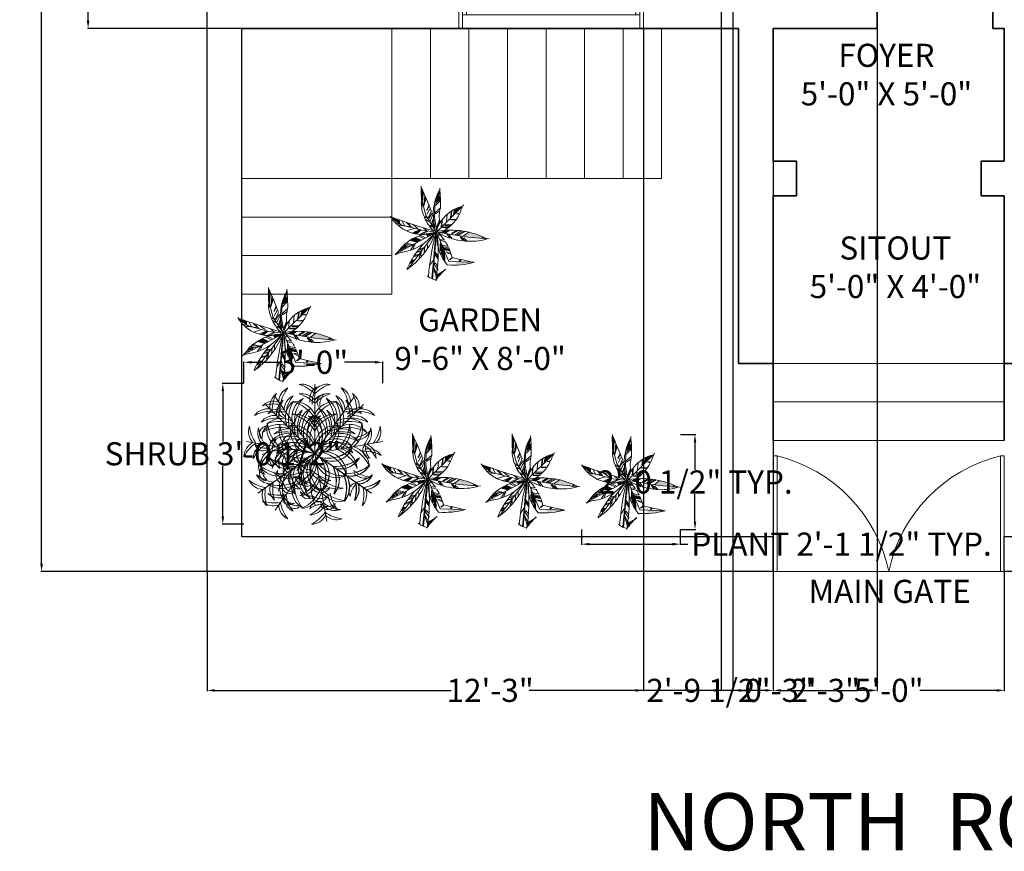
# Model space of a CAD drawing. Units: inches. Extents: x 84 to 590, y 32 to 648.
# Tile 1 of 6: x 84 to 340, y 32 to 248. Entities that reach past the tile are written whole.
import ezdxf

# ---------------------------------------------------------------- set-up
doc = ezdxf.new("R2010")
doc.units = ezdxf.units.IN
doc.header["$MEASUREMENT"] = 0
for name, color, linetype, lineweight in [('A-ANNO-DIMS', 2, 'Continuous', 18), ('A-ANNO-TEXT', 7, 'Continuous', 18), ('A-AREA-IDEN', 7, 'Continuous', 18), ('A-DOOR', 4, 'Continuous', 18), ('A-FLOR-STRS', 7, 'Continuous', 18), ('A-GLAZ', 4, 'Continuous', 18), ('A-WALL', 7, 'Continuous', 35), ('C-PROP', 7, 'Continuous', 30), ('L-PLNT', 3, 'Continuous', 13)]:
    doc.layers.add(name, color=color, linetype=linetype, lineweight=lineweight)
doc.styles.get("Standard").update_dxf_attribs({"font": 'arial.ttf'})
doc.dimstyles.get("Standard").update_dxf_attribs({"dimtxt": 6, "dimasz": 2, "dimexe": 0.18, "dimexo": 0.0625, "dimgap": 0.09, "dimtad": 0, "dimtih": 1, "dimtoh": 1, "dimdec": 0, "dimzin": 0, "dimdsep": 46, "dimlunit": 4, "dimtxsty": 'Standard', "dimcen": 0.09, "dimadec": 0, "dimazin": 0, "dimtfac": 1, "dimtdec": 0, "dimtofl": 0, "dimtmove": 0, "dimatfit": 3, "dimfxl": 1, "dimtolj": 1, "dimtzin": 0, "dimarcsym": 1})

# ---------------------------------------------------------------- blocks, each defined once
blk = doc.blocks.new('DOOR')
for p, q in [((185.51, 1128.53), (185.51, 1098.53)), ((185.51, 1128.53), (186.51, 1128.53)), ((186.51, 1098.53), (186.51, 1128.53)), ((186.51, 1098.53), (156.51, 1098.53))]:
    blk.add_line(p, q)
blk.add_arc((194.73, 1090.6), 39.03, 103.6607, 168.2814)
blk = doc.blocks.new('A$C5D061C3B')
for p, q in [((3.377, 6.679), (3.377, 3.377)), ((1.03, 5.716), (3.365, 3.381)), ((1.483, 6.082), (3.377, 3.377)), ((5.259, 6.086), (3.365, 3.381)), ((5.712, 5.712), (3.377, 3.377)), ((0.125, 3.951), (3.377, 3.377)), ((6.629, 3.951), (3.377, 3.377)), ((0.66, 1.487), (3.365, 3.381)), ((1.483, 0.672), (3.377, 3.377)), ((6.07, 1.487), (3.365, 3.381)), ((3.951, 0.125), (3.377, 3.377)), ((6.082, 1.483), (3.377, 3.377))]:
    blk.add_line(p, q)
for centre, radius, start, end in [((2.763, 5.924), 0.762, 36.29, 99.6243), ((2.145, 5.032), 1.715, 44.0763, 73.3794), ((3.991, 5.924), 0.762, 80.3757, 143.71), ((4.61, 5.032), 1.715, 106.6206, 135.9237), ((1.998, 5.617), 0.762, 125.3757, 188.71), ((3.066, 5.423), 1.715, 151.6206, 180.9237), ((2.419, 5.816), 0.762, 115.3757, 178.71), ((3.438, 5.44), 1.715, 141.6206, 170.9237), ((2.678, 5.447), 0.762, 115.3757, 178.71), ((3.696, 5.07), 1.715, 141.6206, 170.9237), ((2.763, 5.474), 0.762, 36.29, 99.6243), ((2.145, 4.581), 1.715, 44.0763, 73.3794), ((3.901, 5.939), 0.762, 125.3757, 188.71), ((4.969, 5.745), 1.715, 151.6206, 180.9237), ((3.991, 5.474), 0.762, 80.3757, 143.71), ((4.61, 4.581), 1.715, 106.6206, 135.9237), ((3.871, 5.832), 0.38, 94.742, 213.7475), ((4.447, 5.681), 0.826, 139.618, 183.2106), ((4.064, 5.451), 0.762, 1.29, 64.6243), ((3.046, 5.075), 1.715, 9.0763, 38.3794), ((3.305, 5.444), 1.715, 9.0763, 38.3794), ((4.323, 5.82), 0.762, 1.29, 64.6243), ((4.744, 5.613), 0.762, 351.29, 54.6243), ((3.676, 5.419), 1.715, 359.0763, 28.3794), ((1.413, 5.111), 0.762, 71.29, 134.6243), ((1.419, 4.026), 1.715, 79.0763, 108.3794), ((2.317, 5.298), 0.762, 125.3757, 188.71), ((1.991, 5.462), 0.38, 139.742, 258.7475), ((3.385, 5.104), 1.715, 151.6206, 180.9237), ((2.505, 5.763), 0.826, 184.618, 228.2106), ((3.035, 5.062), 1.056, 129.6063, 199.7511), ((3.894, 4.989), 1.77, 149.9634, 193.6288), ((3.344, 5.089), 1.056, 119.6063, 189.7511), ((2.422, 4.799), 1.056, 25.2489, 95.3937), ((1.866, 4.14), 1.77, 31.3712, 75.0366), ((4.177, 4.869), 1.77, 139.9634, 183.6288), ((4.332, 4.799), 1.056, 84.6063, 154.7511), ((4.888, 4.14), 1.77, 104.9634, 148.6288), ((3.398, 5.094), 1.056, 350.2489, 60.3937), ((2.565, 4.873), 1.77, 356.3712, 40.0366), ((2.848, 4.985), 1.77, 346.3712, 30.0366), ((3.707, 5.058), 1.056, 340.2489, 50.3937), ((3.357, 5.1), 1.715, 359.0763, 28.3794), ((4.425, 5.294), 0.762, 351.29, 54.6243), ((1.13, 4.748), 0.762, 81.29, 144.6243), ((1.324, 3.68), 1.715, 89.0763, 118.3794), ((1.448, 4.43), 0.762, 81.29, 144.6243), ((1.671, 4.742), 0.762, 71.29, 134.6243), ((1.677, 3.657), 1.715, 79.0763, 108.3794), ((2.422, 4.198), 1.056, 25.2489, 95.3937), ((1.866, 3.54), 1.77, 31.3712, 75.0366), ((3.46, 4.637), 1.056, 129.6063, 199.7511), ((4.319, 4.565), 1.77, 149.9634, 193.6288), ((3.688, 4.597), 1.056, 119.6063, 189.7511), ((4.522, 4.377), 1.77, 139.9634, 183.6288), ((3.868, 4.321), 1.029, 121.3654, 221.5741), ((4.556, 4.237), 1.557, 141.8122, 203.3335), ((4.035, 4.215), 1.029, 111.3654, 211.5741), ((2.707, 4.219), 1.029, 328.4259, 68.6346), ((2.044, 4.017), 1.557, 346.6665, 48.1878), ((4.698, 4.013), 1.557, 131.8122, 193.3335), ((4.332, 4.198), 1.056, 84.6063, 154.7511), ((4.888, 3.54), 1.77, 104.9634, 148.6288), ((2.187, 4.233), 1.557, 336.6665, 38.1878), ((2.875, 4.316), 1.029, 318.4259, 58.6346), ((2.221, 4.381), 1.77, 356.3712, 40.0366), ((3.054, 4.602), 1.056, 350.2489, 60.3937), ((3.283, 4.633), 1.056, 340.2489, 50.3937), ((2.424, 4.56), 1.77, 346.3712, 30.0366), ((5.065, 3.661), 1.715, 71.6206, 100.9237), ((5.071, 4.746), 0.762, 45.3757, 108.71), ((5.564, 4.807), 0.762, 80.3757, 143.71), ((6.182, 3.914), 1.715, 106.6206, 135.9237), ((5.294, 4.425), 0.762, 35.3757, 98.71), ((5.419, 3.676), 1.715, 61.6206, 90.9237), ((5.613, 4.744), 0.762, 35.3757, 98.71), ((1.642, 3.362), 1.715, 89.0763, 118.3794), ((1.685, 3.712), 1.056, 70.2489, 140.3937), ((2.143, 4.564), 1.056, 164.6063, 234.7511), ((1.78, 3.994), 1.056, 60.2489, 130.3937), ((1.702, 3.136), 1.77, 66.3712, 110.0366), ((2.888, 4.998), 1.77, 184.9634, 228.6288), ((2.734, 4.46), 1.056, 164.6063, 234.7511), ((3.48, 4.893), 1.77, 184.9634, 228.6288), ((2.358, 3.686), 1.029, 3.4259, 103.6346), ((3.25, 4.435), 1.029, 156.3654, 256.5741), ((3.862, 4.761), 1.557, 176.8122, 238.3335), ((4.397, 3.686), 1.029, 76.3654, 176.5741), ((2.893, 4.761), 1.557, 301.6665, 3.1878), ((3.504, 4.435), 1.029, 283.4259, 23.6346), ((5.04, 3.14), 1.77, 69.9634, 113.6288), ((4.963, 3.998), 1.056, 49.6063, 119.7511), ((3.275, 4.893), 1.77, 311.3712, 355.0366), ((4.02, 4.46), 1.056, 305.2489, 15.3937), ((5.058, 3.707), 1.056, 39.6063, 109.7511), ((3.866, 4.998), 1.77, 311.3712, 355.0366), ((5.1, 3.357), 1.715, 61.6206, 90.9237), ((4.611, 4.564), 1.056, 305.2489, 15.3937), ((0.975, 4.424), 0.762, 160.3757, 223.71), ((1.962, 4.878), 1.715, 186.6206, 215.9237), ((1.419, 4.346), 0.762, 160.3757, 223.71), ((2.405, 4.8), 1.715, 186.6206, 215.9237), ((1.12, 4.31), 0.38, 94.742, 213.7475), ((1.696, 4.159), 0.826, 139.618, 183.2106), ((1.757, 2.853), 1.77, 76.3712, 120.0366), ((2.109, 3.287), 1.056, 70.2489, 140.3937), ((2.124, 3.502), 1.056, 60.2489, 130.3937), ((2.046, 2.644), 1.77, 66.3712, 110.0366), ((2.387, 3.752), 0.574, 99.9865, 199.4034), ((3.599, 3.314), 1.651, 142.5759, 170.8942), ((1.93, 3.14), 1.557, 21.6665, 83.1878), ((4.824, 3.14), 1.557, 96.8122, 158.3335), ((4.696, 2.648), 1.77, 69.9634, 113.6288), ((4.618, 3.506), 1.056, 49.6063, 119.7511), ((4.633, 3.283), 1.056, 39.6063, 109.7511), ((4.985, 2.848), 1.77, 59.9634, 103.6288), ((4.988, 5.812), 1.715, 279.0763, 308.3794), ((5.365, 4.794), 0.762, 271.29, 334.6243), ((4.349, 4.8), 1.715, 324.0763, 353.3794), ((5.335, 4.346), 0.762, 316.29, 19.6243), ((4.793, 4.878), 1.715, 324.0763, 353.3794), ((5.779, 4.424), 0.762, 316.29, 19.6243), ((0.762, 3.214), 0.762, 116.29, 179.6243), ((1.534, 2.451), 1.715, 124.0763, 153.3794), ((1.206, 3.136), 0.762, 116.29, 179.6243), ((1.977, 2.373), 1.715, 124.0763, 153.3794), ((1.062, 4.452), 0.826, 229.618, 273.2106), ((0.91, 3.875), 0.38, 184.742, 303.7475), ((1.588, 3.666), 0.38, 94.742, 213.7475), ((2.182, 2.428), 1.77, 76.3712, 120.0366), ((2.165, 3.515), 0.826, 139.618, 183.2106), ((2.426, 2.879), 1.029, 48.4259, 148.6346), ((2.365, 3.045), 1.029, 38.4259, 138.6346), ((2.328, 2.353), 1.557, 56.6665, 118.1878), ((2.84, 3.739), 0.372, 69.2257, 210.1279), ((3.109, 3.59), 0.515, 105.4398, 183.6694), ((4.414, 2.358), 1.557, 61.8122, 123.3335), ((4.377, 3.05), 1.029, 41.3654, 141.5741), ((4.316, 2.875), 1.029, 31.3654, 131.5741), ((4.56, 2.424), 1.77, 59.9634, 103.6288), ((4.777, 2.373), 1.715, 26.6206, 55.9237), ((5.549, 3.136), 0.762, 0.3757, 63.71), ((1.811, 2.684), 1.056, 105.2489, 175.3937), ((2.363, 2.022), 1.77, 111.3712, 155.0366), ((2.185, 0.015), 3.567, 70.4772, 111.6585), ((1.447, 3.129), 0.376, 122.0577, 257.8533), ((1.751, 3.126), 0.529, 140.1845, 223.654), ((2.403, 2.58), 1.056, 105.2489, 175.3937), ((2.955, 1.917), 1.77, 111.3712, 155.0366), ((2.007, 3.071), 0.506, 93.8744, 233.9763), ((2.51, 2.191), 1.557, 66.6665, 128.1878), ((2.729, 4.702), 1.557, 221.8122, 283.3335), ((2.527, 4.039), 1.029, 201.3654, 301.5741), ((4.912, 0.157), 3.567, 115.4772, 156.6585), ((2.489, 2.932), 0.825, 128.7536, 199.097), ((2.896, 2.427), 1.029, 83.4259, 183.6346), ((3.359, 1.911), 1.557, 101.6665, 163.1878), ((2.903, 2.8), 0.855, 116.4477, 194.3672), ((4.744, 1.779), 2.789, 140.4007, 163.139), ((2.741, 3.253), 0.372, 114.2257, 255.1279), ((3.037, 3.338), 0.515, 150.4398, 228.6694), ((6.727, 2.189), 3.567, 160.4772, 201.6585), ((4.233, 2.187), 1.557, 51.8122, 113.3335), ((4.001, 4.702), 1.557, 256.6665, 318.1878), ((4.013, 4.698), 1.557, 256.6665, 318.1878), ((4.203, 4.039), 1.029, 238.4259, 338.6346), ((4.215, 4.035), 1.029, 238.4259, 338.6346), ((3.395, 1.911), 1.557, 16.8122, 78.3335), ((3.858, 2.427), 1.029, 356.3654, 96.5741), ((3.799, 1.917), 1.77, 24.9634, 68.6288), ((4.352, 2.58), 1.056, 4.6063, 74.7511), ((4.391, 2.022), 1.77, 24.9634, 68.6288), ((4.943, 2.684), 1.056, 4.6063, 74.7511), ((6.053, 3.533), 0.38, 146.2525, 265.258), ((5.741, 1.774), 1.715, 61.6206, 90.9237), ((6.629, 3.684), 0.826, 176.7894, 220.382), ((5.935, 2.842), 0.762, 35.3757, 98.71), ((1.067, 2.749), 0.376, 122.0577, 257.8533), ((1.873, 4.181), 1.77, 229.9634, 273.6288), ((1.653, 3.348), 1.056, 209.6063, 279.7511), ((1.37, 2.745), 0.529, 140.1845, 223.654), ((2.145, 3.693), 1.056, 209.6063, 279.7511), ((2.365, 4.526), 1.77, 229.9634, 273.6288), ((2.328, 4.401), 1.557, 241.8122, 303.3335), ((2.365, 3.709), 1.029, 221.3654, 321.5741), ((2.412, 2.943), 0.574, 144.9865, 244.4034), ((3.578, 3.49), 1.651, 187.5759, 215.8942), ((1.911, 3.359), 1.557, 286.8122, 348.3335), ((2.427, 2.896), 1.029, 266.3654, 6.5741), ((3.45, 2.634), 0.855, 161.4477, 239.3672), ((3.003, 2.844), 0.372, 159.2257, 300.1279), ((3.152, 3.113), 0.515, 195.4398, 273.6694), ((3.697, 2.369), 1.029, 128.4259, 228.6346), ((5.474, 3.214), 2.789, 185.4007, 208.139), ((4.389, 2.332), 1.557, 146.6665, 208.1878), ((4.035, 2.539), 1.029, 148.4259, 248.6346), ((4.698, 2.741), 1.557, 166.6665, 228.1878), ((4.435, 3.25), 1.029, 193.4259, 293.6346), ((4.761, 3.862), 1.557, 211.6665, 273.1878), ((2.341, 2.332), 1.557, 331.8122, 33.3335), ((2.353, 2.328), 1.557, 331.8122, 33.3335), ((3.033, 2.369), 1.029, 311.3654, 51.5741), ((3.045, 2.365), 1.029, 311.3654, 51.5741), ((4.365, 4.526), 1.77, 266.3712, 310.0366), ((4.377, 4.522), 1.77, 266.3712, 310.0366), ((4.585, 3.693), 1.056, 260.2489, 330.3937), ((4.597, 3.688), 1.056, 260.2489, 330.3937), ((4.857, 4.181), 1.77, 266.3712, 310.0366), ((4.869, 4.177), 1.77, 266.3712, 310.0366), ((5.077, 3.348), 1.056, 260.2489, 330.3937), ((5.089, 3.344), 1.056, 260.2489, 330.3937), ((1.672, 3.7), 1.715, 231.6206, 260.9237), ((1.295, 2.682), 0.762, 205.3757, 268.71), ((1.122, 2.441), 0.38, 139.742, 258.7475), ((1.636, 2.741), 0.826, 184.618, 228.2106), ((2.046, 4.111), 1.77, 249.9634, 293.6288), ((2.124, 3.252), 1.056, 229.6063, 299.7511), ((1.908, 2.317), 0.38, 139.742, 258.7475), ((2.422, 2.617), 0.826, 184.618, 228.2106), ((3.607, 1.706), 1.77, 156.3712, 200.0366), ((2.624, 2.192), 0.506, 138.8744, 278.9763), ((3.24, 2.128), 1.056, 150.2489, 220.3937), ((3.064, 2.435), 0.825, 173.7536, 244.097), ((4.099, 2.051), 1.77, 156.3712, 200.0366), ((4.522, 2.378), 1.77, 176.3712, 220.0366), ((3.942, 2.908), 0.855, 206.4477, 284.3672), ((4.963, 4.749), 2.789, 230.4007, 253.139), ((2.632, 2.051), 1.77, 339.9634, 23.6288), ((2.644, 2.046), 1.77, 339.9634, 23.6288), ((3.49, 2.128), 1.056, 319.6063, 29.7511), ((3.502, 2.124), 1.056, 319.6063, 29.7511), ((3.124, 1.706), 1.77, 339.9634, 23.6288), ((3.136, 1.702), 1.77, 339.9634, 23.6288), ((6.244, 3.948), 1.715, 234.0763, 263.3794), ((5.79, 2.962), 0.762, 226.29, 289.6243), ((5.058, 3.7), 1.715, 279.0763, 308.3794), ((5.07, 3.696), 1.715, 279.0763, 308.3794), ((5.435, 2.682), 0.762, 271.29, 334.6243), ((5.447, 2.678), 0.762, 271.29, 334.6243), ((0.926, 2.424), 0.762, 205.3757, 268.71), ((1.303, 3.442), 1.715, 231.6206, 260.9237), ((1.702, 3.619), 1.77, 249.9634, 293.6288), ((1.78, 2.76), 1.056, 229.6063, 299.7511), ((2, 1.676), 0.762, 161.29, 224.6243), ((3.086, 1.681), 1.715, 169.0763, 198.3794), ((2.748, 1.784), 1.056, 150.2489, 220.3937), ((2.188, 1.837), 0.376, 167.0577, 302.8533), ((2.405, 2.049), 0.529, 185.1845, 268.654), ((4.177, 1.886), 1.77, 176.3712, 220.0366), ((3.428, 3.603), 1.651, 232.5759, 260.8942), ((2.99, 2.391), 0.574, 189.9865, 289.4034), ((3.688, 2.157), 1.056, 170.2489, 240.3937), ((1.917, 2.955), 1.77, 294.9634, 338.6288), ((2.58, 2.403), 1.056, 274.6063, 344.7511), ((3.81, 2.493), 0.825, 218.7536, 289.097), ((3.671, 2.011), 0.506, 183.8744, 323.9763), ((4.893, 3.48), 1.77, 221.3712, 265.0366), ((4.46, 2.734), 1.056, 215.2489, 285.3937), ((3.982, 1.784), 1.056, 319.6063, 29.7511), ((3.994, 1.78), 1.056, 319.6063, 29.7511), ((5.385, 1.584), 0.38, 101.2525, 220.258), ((5.899, 1.283), 0.826, 131.7894, 175.382), ((3.645, 1.681), 1.715, 341.6206, 10.9237), ((4.73, 1.676), 0.762, 315.3757, 18.71), ((3.657, 1.677), 1.715, 341.6206, 10.9237), ((4.742, 1.671), 0.762, 315.3757, 18.71), ((5.427, 3.442), 1.715, 279.0763, 308.3794), ((5.44, 3.438), 1.715, 279.0763, 308.3794), ((5.804, 2.424), 0.762, 271.29, 334.6243), ((5.816, 2.419), 0.762, 271.29, 334.6243), ((1.631, 1.417), 0.762, 161.29, 224.6243), ((2.717, 1.423), 1.715, 169.0763, 198.3794), ((1.671, 2.012), 0.762, 225.3757, 288.71), ((1.677, 3.098), 1.715, 251.6206, 280.9237), ((2.405, 1.511), 0.529, 185.1845, 268.654), ((3.696, 1.684), 1.715, 189.0763, 218.3794), ((3.344, 1.665), 1.056, 170.2489, 240.3937), ((3.227, 2.169), 0.826, 229.618, 273.2106), ((3.076, 1.593), 0.38, 184.742, 303.7475), ((2.022, 2.363), 1.77, 294.9634, 338.6288), ((2.684, 1.811), 1.056, 274.6063, 344.7511), ((4.998, 2.888), 1.77, 221.3712, 265.0366), ((4.564, 2.143), 1.056, 215.2489, 285.3937), ((5.808, 1.754), 1.715, 189.0763, 218.3794), ((4.014, 1.423), 1.715, 341.6206, 10.9237), ((5.099, 1.417), 0.762, 315.3757, 18.71), ((1.419, 2.729), 1.715, 251.6206, 280.9237), ((1.413, 1.643), 0.762, 225.3757, 288.71), ((3.438, 1.315), 1.715, 189.0763, 218.3794), ((2.188, 1.299), 0.376, 167.0577, 302.8533), ((2.678, 1.307), 0.762, 181.29, 244.6243), ((2.583, 1.701), 0.826, 229.618, 273.2106), ((2.432, 1.124), 0.38, 184.742, 303.7475), ((2.373, 1.977), 1.715, 296.6206, 325.9237), ((3.528, 0.69), 0.38, 56.2525, 175.258), ((3.616, 1.755), 0.529, 230.1845, 313.654), ((3.613, 1.452), 0.376, 212.0577, 347.8533), ((3.997, 1.374), 0.529, 230.1845, 313.654), ((3.994, 1.071), 0.376, 212.0577, 347.8533), ((4.8, 2.405), 1.715, 234.0763, 263.3794), ((4.79, 1.377), 0.762, 181.29, 244.6243), ((2.419, 0.938), 0.762, 181.29, 244.6243), ((3.136, 1.206), 0.762, 270.3757, 333.71), ((3.68, 0.113), 0.826, 86.7894, 130.382), ((2.451, 1.534), 1.715, 296.6206, 325.9237), ((4.346, 1.419), 0.762, 226.29, 289.6243), ((4.878, 1.962), 1.715, 234.0763, 263.3794), ((3.214, 0.762), 0.762, 270.3757, 333.71), ((4.424, 0.975), 0.762, 226.29, 289.6243)]:
    blk.add_arc(centre, radius, start, end)
blk = doc.blocks.new('A$C40F70BF2')
for p, q in [((1.395, 3.412), (1.345, 4.14)), ((1.378, 3.827), (1.371, 4.019)), ((1.386, 3.761), (1.393, 4.004)), ((1.404, 3.622), (1.407, 3.935)), ((1.411, 3.538), (1.419, 3.905)), ((1.937, 3.412), (2.147, 3.983)), ((2.077, 3.788), (2.151, 3.896)), ((1.389, 3.49), (1.353, 3.553)), ((1.393, 3.445), (1.356, 3.526)), ((1.393, 3.403), (1.356, 3.493)), ((1.411, 3.334), (1.36, 3.445)), ((1.448, 3.313), (1.496, 3.752)), ((1.529, 3.679), (1.455, 3.289)), ((1.455, 3.289), (1.55, 3.622)), ((2.18, 3.523), (1.96, 3.294)), ((1.974, 3.403), (2.165, 3.619)), ((2.165, 3.571), (1.974, 3.403)), ((1.989, 3.487), (2.151, 3.679)), ((2.165, 3.619), (1.989, 3.487)), ((2.033, 3.595), (2.135, 3.727)), ((2.151, 3.679), (2.033, 3.595)), ((2.062, 3.679), (2.135, 3.824)), ((2.135, 3.727), (2.062, 3.679)), ((2.135, 3.824), (2.077, 3.788)), ((1.43, 3.289), (1.349, 3.412)), ((1.426, 3.264), (1.353, 3.376)), ((1.536, 2.871), (1.395, 3.412)), ((1.587, 3.114), (1.683, 3.328)), ((1.591, 3.078), (1.587, 3.114)), ((1.701, 3.289), (1.591, 3.078)), ((1.606, 2.916), (1.705, 3.132)), ((1.65, 2.748), (1.785, 3.066)), ((1.919, 2.785), (1.937, 3.412)), ((1.96, 3.006), (2.18, 3.198)), ((2.151, 3.066), (1.96, 2.933)), ((2.006, 2.139), (3.105, 3.225)), ((2.626, 2.774), (2.662, 3.065)), ((2.653, 2.781), (2.685, 3.069)), ((2.797, 3.138), (2.753, 2.909)), ((2.855, 3.162), (2.797, 2.933)), ((2.797, 2.933), (2.797, 3.138)), ((2.885, 3.162), (2.826, 2.957)), ((2.826, 2.957), (2.855, 3.162)), ((2.929, 3.174), (2.855, 3.006)), ((2.855, 3.006), (2.885, 3.162)), ((2.899, 3.018), (2.929, 3.174)), ((2.944, 3.15), (2.899, 3.018)), ((2.958, 3.186), (2.929, 3.066)), ((2.929, 3.066), (2.944, 3.15)), ((2.973, 3.114), (2.958, 3.186)), ((3.002, 3.21), (2.973, 3.114)), ((3.032, 3.234), (3.002, 3.162)), ((3.002, 3.162), (3.002, 3.21)), ((0.438, 2.456), (0.018, 2.796)), ((0.505, 2.608), (0.623, 2.404)), ((1.58, 2.772), (1.451, 2.841)), ((1.472, 2.791), (1.602, 2.739)), ((1.992, 2.139), (1.536, 2.871)), ((1.538, 2.69), (1.679, 2.617)), ((1.564, 2.648), (1.679, 2.596)), ((1.602, 2.739), (1.58, 2.772)), ((1.668, 2.733), (1.65, 2.748)), ((1.822, 2.967), (1.668, 2.733)), ((1.73, 2.628), (1.844, 2.883)), ((1.789, 2.517), (1.873, 2.748)), ((1.8, 2.478), (1.88, 2.664)), ((2.024, 2.154), (1.919, 2.785)), ((1.96, 2.933), (1.96, 3.006)), ((2.216, 2.359), (2.243, 2.624)), ((2.238, 2.386), (2.257, 2.647)), ((2.446, 2.617), (2.471, 2.889)), ((2.621, 2.684), (2.895, 2.703)), ((2.621, 2.677), (2.849, 2.673)), ((2.877, 2.934), (3.045, 2.983)), ((3.008, 2.919), (2.877, 2.934)), ((0.211, 2.512), (0.476, 2.476)), ((0.314, 2.44), (0.828, 2.38)), ((1.381, 2.214), (0.438, 2.456)), ((0.696, 2.548), (0.916, 2.356)), ((0.696, 2.187), (1.034, 2.295)), ((0.916, 2.356), (0.784, 2.5)), ((0.96, 2.476), (1.196, 2.295)), ((1.269, 2.236), (0.96, 2.103)), ((1.019, 2.067), (1.269, 2.236)), ((1.078, 2.062), (1.295, 2.219)), ((1.129, 2.052), (1.321, 2.219)), ((1.313, 2.055), (1.578, 2.175)), ((1.974, 2.139), (1.381, 2.214)), ((1.387, 2.043), (1.665, 2.187)), ((1.431, 2.32), (1.592, 2.199)), ((1.789, 2.411), (1.627, 2.469)), ((1.672, 2.415), (1.811, 2.369)), ((1.811, 2.369), (1.789, 2.411)), ((2.27, 2.33), (2.289, 2.356)), ((2.498, 2.311), (2.27, 2.33)), ((2.289, 2.356), (2.58, 2.344)), ((2.366, 2.415), (2.384, 2.442)), ((2.612, 2.4), (2.366, 2.415)), ((2.369, 2.481), (2.676, 2.471)), ((2.375, 2.079), (2.567, 2.21)), ((2.384, 2.442), (2.644, 2.427)), ((2.662, 2.072), (2.881, 2.203)), ((2.699, 2.053), (2.968, 2.206)), ((2.831, 2.016), (3.118, 2.199)), ((2.913, 2.012), (3.218, 2.176)), ((3.264, 2.165), (2.977, 2.001)), ((1.974, 2.113), (0.228, 1.183)), ((1.974, 2.128), (0.802, 0.571)), ((1.225, 1.959), (1.46, 1.862)), ((1.284, 2.007), (1.504, 1.898)), ((2.003, 2.103), (1.827, 0.082)), ((1.974, 1.995), (1.915, 1.405)), ((2.006, 2.139), (2.548, 0.855)), ((2.07, 2.139), (2.758, 2.02)), ((2.083, 2.012), (2.22, 1.967)), ((2.179, 1.762), (2.156, 1.818)), ((2.156, 1.818), (2.361, 1.788)), ((2.402, 1.714), (2.179, 1.762)), ((2.548, 2.035), (2.457, 2.046)), ((2.457, 2.046), (2.603, 1.863)), ((2.69, 1.84), (2.548, 2.035)), ((2.758, 2.02), (3.387, 1.915)), ((2.977, 2.001), (2.913, 2.012)), ((3.177, 1.747), (3.041, 1.93)), ((3.041, 1.93), (3.105, 1.915)), ((3.105, 1.915), (3.255, 1.736)), ((3.168, 1.952), (3.415, 2.135)), ((3.332, 1.747), (3.196, 1.889)), ((3.387, 1.915), (3.907, 1.867)), ((3.911, 1.863), (4.308, 1.837)), ((3.975, 1.885), (4.057, 1.915)), ((4.012, 1.878), (3.975, 1.885)), ((4.085, 1.904), (4.012, 1.878)), ((0.387, 1.333), (0.505, 1.357)), ((0.417, 1.381), (0.578, 1.405)), ((0.505, 1.357), (0.417, 1.381)), ((0.461, 1.429), (0.667, 1.442)), ((0.578, 1.405), (0.461, 1.429)), ((0.476, 1.465), (0.696, 1.478)), ((0.667, 1.442), (0.476, 1.465)), ((0.696, 1.478), (0.549, 1.526)), ((0.549, 1.526), (0.814, 1.513)), ((0.814, 1.513), (0.578, 1.562)), ((0.593, 1.61), (0.902, 1.562)), ((0.96, 1.586), (0.667, 1.646)), ((0.872, 1.345), (1.019, 1.586)), ((0.902, 1.562), (0.96, 1.586)), ((0.989, 1.405), (1.093, 1.646)), ((1.206, 1.34), (1.436, 1.403)), ((1.231, 1.403), (1.462, 1.445)), ((1.475, 1.237), (1.504, 1.501)), ((1.915, 1.405), (1.871, 0.852)), ((2.175, 1.512), (2.165, 1.441)), ((2.165, 1.441), (2.165, 1.363)), ((2.179, 1.676), (2.175, 1.605)), ((2.175, 1.605), (2.175, 1.512)), ((2.179, 1.314), (2.179, 1.676)), ((2.184, 1.501), (2.179, 1.407)), ((2.179, 1.407), (2.179, 1.314)), ((2.193, 1.613), (2.184, 1.501)), ((2.197, 1.46), (2.193, 1.613)), ((2.197, 1.392), (2.197, 1.46)), ((2.206, 1.277), (2.197, 1.392)), ((2.225, 1.501), (2.211, 1.378)), ((2.211, 1.378), (2.211, 1.172)), ((2.216, 1.34), (2.225, 1.422)), ((2.216, 1.273), (2.216, 1.34)), ((2.225, 1.422), (2.225, 1.501)), ((2.238, 1.303), (2.229, 1.232)), ((2.243, 1.389), (2.238, 1.303)), ((2.247, 1.46), (2.243, 1.389)), ((2.257, 1.534), (2.247, 1.46)), ((2.257, 1.544), (2.257, 1.534)), ((2.261, 1.213), (2.261, 1.535)), ((2.298, 1.486), (2.27, 1.56)), ((2.27, 1.56), (2.521, 1.501)), ((2.279, 1.396), (2.275, 1.314)), ((2.275, 1.314), (2.275, 1.247)), ((2.289, 1.318), (2.279, 1.396)), ((2.289, 1.157), (2.289, 1.318)), ((2.302, 1.292), (2.293, 1.224)), ((2.548, 1.441), (2.298, 1.486)), ((2.307, 1.37), (2.302, 1.292)), ((2.307, 1.023), (2.307, 1.37)), ((2.334, 0.926), (2.343, 1.325)), ((2.371, 0.847), (2.357, 1.299)), ((0.843, 0.792), (0.989, 0.876)), ((0.872, 0.864), (1.049, 0.924)), ((0.989, 0.876), (0.872, 0.864)), ((1.049, 0.924), (0.931, 0.912)), ((1.019, 1.056), (1.21, 1.129)), ((1.049, 1.105), (1.24, 1.165)), ((1.254, 1.008), (1.313, 1.249)), ((1.327, 1.093), (1.342, 1.273)), ((1.709, 0.671), (1.871, 0.912)), ((1.944, 1.141), (1.944, 1.261)), ((1.944, 1.261), (2.077, 1.08)), ((2.077, 0.948), (1.944, 1.141)), ((2.062, 1.026), (1.947, 1.204)), ((2.206, 1.105), (2.206, 1.277)), ((2.211, 1.172), (2.206, 1.105)), ((2.225, 1.157), (2.216, 1.273)), ((2.229, 1.232), (2.225, 1.157)), ((2.27, 1.109), (2.261, 1.213)), ((2.275, 1.247), (2.27, 1.18)), ((2.27, 1.18), (2.27, 1.109)), ((2.293, 1.015), (2.289, 1.157)), ((2.293, 1.154), (2.289, 1.083)), ((2.289, 1.083), (2.293, 1.015)), ((2.293, 1.224), (2.293, 1.154)), ((2.311, 0.948), (2.307, 1.023)), ((2.433, 1.267), (2.637, 1.215)), ((2.471, 1.236), (2.65, 1.152)), ((2.69, 1.027), (2.571, 0.922)), ((2.699, 1.008), (2.594, 0.922)), ((3.063, 0.941), (2.995, 0.87)), ((3.095, 0.937), (3.013, 0.851)), ((0.814, 0.744), (0.96, 0.804)), ((0.96, 0.804), (0.843, 0.792)), ((1.871, 0.852), (1.798, 0.13)), ((1.886, 0.527), (1.886, 0.587)), ((1.886, 0.587), (2.003, 0.322)), ((2.003, 0.154), (1.886, 0.527)), ((1.915, 0.696), (1.93, 0.792)), ((2.077, 0.491), (1.915, 0.696)), ((1.93, 0.792), (2.062, 0.647)), ((2.548, 0.855), (3.647, 0.814))]:
    blk.add_line(p, q)
for centre, radius, start, end in [((7.228, 3.925), 5.886, 178.201, 184.8569), ((-12.631, -2.337), 15.387, 20.511, 24.7274), ((3.986, 2.93), 2.121, 151.1341, 194.9744), ((-4.468, 3.341), 6.654, 358.6497, 6.1521), ((3.081, 3.443), 1.737, 181.0191, 200.3048), ((3.488, 1.763), 1.537, 103.7474, 164.6646), ((3.323, 2.824), 1.195, 162.4534, 194.3671), ((1.484, 3.655), 1.692, 336.4968, 341.7386), ((4.255, 2.671), 1.249, 148.3784, 158.7208), ((1.388, 3.636), 1.607, 210.2718, 288.6073), ((11.205, 34.008), 33.156, 250.2818, 253.6131), ((3.081, 3.443), 1.737, 202.0613, 214.4357), ((-12.631, -2.337), 15.387, 19.9468, 20.1294), ((1.484, 3.655), 1.692, 293.0839, 334.2208), ((3.081, 3.443), 1.737, 216.4922, 227.1869), ((2.648, -1.238), 3.457, 62.9286, 99.782), ((1.97, 0.03), 2.073, 93.8052, 134.9428), ((0.206, 3.365), 2.134, 278.5823, 322.5951), ((-1.258, 3.332), 3.452, 304.8805, 336.243), ((14.63, -0.992), 13.028, 166.2796, 174.8216), ((-5.402, 1.247), 7.481, 350.4062, 5.6425), ((3.808, 1.866), 1.768, 177.0625, 221.9788), ((0.371, 0.432), 2.394, 34.5841, 45.0988), ((3.478, 4.556), 2.822, 241.8528, 251.6799), ((3.478, 4.556), 2.822, 253.6434, 263.8215), ((3.478, 4.556), 2.822, 265.3232, 284.5956), ((-1.183, 2.66), 2.05, 312.2483, 325.4397), ((4.234, -0.992), 3.827, 137.0982, 156.8626), ((0.371, 0.432), 2.394, 26.5664, 32.4272), ((0.371, 0.432), 2.394, 14.3751, 24.9555), ((0.622, 0.416), 0.842, 95.4287, 120.3984), ((10.9, 35.08), 35.029, 256.4454, 258.0204), ((5.057, -2.3), 3.867, 133.3547, 142.8755), ((1.268, 2.121), 1.986, 292.1292, 305.3212), ((2.731, 4.141), 3.451, 266.0609, 285.3989), ((2.112, 0.756), 0.732, 226.5793, 260.5482)]:
    blk.add_arc(centre, radius, start, end)
for points in [[(0.035, 2.801), (0.417, 2.5), (0.035, 2.801), (0.402, 2.657)], [(1.983, 2.159), (1.888, 2.598), (1.983, 2.159), (1.818, 2.432)], [(2.02, 2.234), (2.16, 2.54), (1.994, 2.357), (2.13, 2.691)], [(2.398, 2.087), (2.562, 2.203), (2.206, 2.12), (2.366, 2.203)], [(1.136, 1.682), (0.828, 1.766), (1.357, 1.79), (1.107, 1.911)], [(1.93, 2.091), (1.607, 1.923), (1.886, 2.091), (1.533, 2.055)], [(2.003, 2.043), (2.062, 1.465), (2.003, 2.031), (1.96, 1.586)], [(3.893, 1.874), (4.007, 1.93), (3.228, 1.952), (3.451, 2.12)], [(1.357, 1.297), (1.078, 1.201), (1.387, 1.357), (1.151, 1.273)], [(1.592, 1.393), (1.592, 1.61), (1.636, 1.478), (1.622, 1.682)], [(2.598, 1.303), (2.343, 1.34), (2.557, 1.407), (2.293, 1.467)], [(2.003, 0.058), (2.385, 0.503), (2.018, 0.286), (2.4, 0.503)], [(3.546, 0.816), (2.811, 0.852), (3.59, 0.804), (2.914, 0.708)]]:
    blk.add_solid(points)
blk = doc.blocks.new('*D13')
at = {"layer": 'A-ANNO-DIMS', "color": 0, "lineweight": -2, "transparency": 16777216}
for p, q in [((132.97, 608.34), (89.87, 608.34)), ((90.05, 606.34), (90.05, 359.49)), ((90.05, 106.34), (90.05, 353.18)), ((132.97, 104.34), (89.87, 104.34))]:
    blk.add_line(p, q, dxfattribs=at)
at = {"layer": 'A-ANNO-DIMS', "color": 0, "transparency": 16777216}
for points in [[(89.71, 606.34), (90.38, 606.34), (90.05, 608.34)], [(89.71, 106.34), (90.38, 106.34), (90.05, 104.34)]]:
    blk.add_solid(points, dxfattribs=at)
at = {"layer": 'Defpoints', "color": 0, "transparency": 16777216}
for p in [(90.05, 608.34), (133.03, 608.34), (133.03, 104.34)]:
    blk.add_point(p, dxfattribs=at)
at = {"layer": 'A-ANNO-DIMS', "color": 0, "transparency": 16777216, "insert": (90.05, 356.34), "char_height": 6, "attachment_point": 5}
blk.add_mtext("\\A1;40'", dxfattribs=at)
blk = doc.blocks.new('WIND')
for p, q in [((-51.89, 1021.98), (-99.89, 1021.98)), ((-99.89, 1021.98), (-99.89, 1012.98)), ((-98.89, 1021.98), (-98.89, 1012.98)), ((-52.89, 1012.98), (-52.89, 1021.98)), ((-51.89, 1012.98), (-51.89, 1021.98)), ((-98.89, 1018.48), (-52.89, 1018.48)), ((-97.89, 1018.48), (-97.89, 1016.48)), ((-53.89, 1016.48), (-53.89, 1018.48)), ((-98.89, 1016.48), (-52.89, 1016.48)), ((-97.89, 1017.48), (-53.89, 1017.48)), ((-99.89, 1012.98), (-51.89, 1012.98))]:
    blk.add_line(p, q)
blk = doc.blocks.new('*D37')
at = {"layer": 'A-ANNO-DIMS', "color": 0, "lineweight": -2, "transparency": 16777216}
for p, q in [((230.27, 115.19), (230.27, 111.23)), ((255.87, 115.19), (255.87, 111.23)), ((232.27, 111.41), (253.87, 111.41)), ((255.87, 111.41), (257.87, 111.41))]:
    blk.add_line(p, q, dxfattribs=at)
at = {"layer": 'A-ANNO-DIMS', "color": 0, "transparency": 16777216}
for points in [[(232.27, 111.74), (232.27, 111.08), (230.27, 111.41)], [(253.87, 111.74), (253.87, 111.08), (255.87, 111.41)]]:
    blk.add_solid(points, dxfattribs=at)
at = {"layer": 'Defpoints', "color": 0, "transparency": 16777216}
for p in [(230.27, 115.25), (255.87, 115.25), (255.87, 111.41)]:
    blk.add_point(p, dxfattribs=at)
at = {"layer": 'A-ANNO-DIMS', "color": 0, "transparency": 16777216, "insert": (297.76, 111.41), "char_height": 6, "attachment_point": 5}
blk.add_mtext('\\A1;PLANT 2\'-1 1/2" TYP.', dxfattribs=at)
blk = doc.blocks.new('*D38')
at = {"layer": 'A-ANNO-DIMS', "color": 0, "lineweight": -2, "transparency": 16777216}
for p, q in [((255.93, 139.85), (259.89, 139.85)), ((259.71, 137.85), (259.71, 130.74)), ((259.71, 117.25), (259.71, 124.36)), ((255.93, 115.25), (259.89, 115.25))]:
    blk.add_line(p, q, dxfattribs=at)
at = {"layer": 'A-ANNO-DIMS', "color": 0, "transparency": 16777216}
for points in [[(259.38, 137.85), (260.04, 137.85), (259.71, 139.85)], [(259.38, 117.25), (260.04, 117.25), (259.71, 115.25)]]:
    blk.add_solid(points, dxfattribs=at)
at = {"layer": 'Defpoints', "color": 0, "transparency": 16777216}
for p in [(255.87, 139.85), (259.71, 139.85), (255.87, 115.25)]:
    blk.add_point(p, dxfattribs=at)
at = {"layer": 'A-ANNO-DIMS', "color": 0, "transparency": 16777216, "insert": (259.71, 127.55), "char_height": 6, "attachment_point": 5}
blk.add_mtext('\\A1;2\'-0 1/2" TYP.', dxfattribs=at)
blk = doc.blocks.new('*D39')
at = {"layer": 'A-ANNO-DIMS', "color": 0, "lineweight": -2, "transparency": 16777216}
for p, q in [((142.53, 153.15), (136.93, 153.15)), ((137.11, 151.15), (137.11, 138.06)), ((137.11, 118.59), (137.11, 131.67)), ((142.53, 116.59), (136.93, 116.59))]:
    blk.add_line(p, q, dxfattribs=at)
at = {"layer": 'A-ANNO-DIMS', "color": 0, "transparency": 16777216}
for points in [[(136.78, 151.15), (137.44, 151.15), (137.11, 153.15)], [(136.78, 118.59), (137.44, 118.59), (137.11, 116.59)]]:
    blk.add_solid(points, dxfattribs=at)
at = {"layer": 'Defpoints', "color": 0, "transparency": 16777216}
for p in [(137.11, 153.15), (142.6, 153.15), (142.6, 116.59)]:
    blk.add_point(p, dxfattribs=at)
at = {"layer": 'A-ANNO-DIMS', "color": 0, "transparency": 16777216, "insert": (137.11, 134.87), "char_height": 6, "attachment_point": 5}
blk.add_mtext('\\A1;SHRUB 3\'-0 1/2"', dxfattribs=at)
blk = doc.blocks.new('*D40')
at = {"layer": 'A-ANNO-DIMS', "color": 0, "lineweight": -2, "transparency": 16777216}
for p, q in [((142.6, 153.21), (142.6, 158.81)), ((144.6, 158.63), (152.56, 158.63)), ((176.64, 158.63), (168.68, 158.63)), ((178.64, 153.21), (178.64, 158.81))]:
    blk.add_line(p, q, dxfattribs=at)
at = {"layer": 'A-ANNO-DIMS', "color": 0, "transparency": 16777216}
for points in [[(144.6, 158.97), (144.6, 158.3), (142.6, 158.63)], [(176.64, 158.97), (176.64, 158.3), (178.64, 158.63)]]:
    blk.add_solid(points, dxfattribs=at)
at = {"layer": 'Defpoints', "color": 0, "transparency": 16777216}
for p in [(178.64, 158.63), (142.6, 153.15), (178.64, 153.15)]:
    blk.add_point(p, dxfattribs=at)
at = {"layer": 'A-ANNO-DIMS', "color": 0, "transparency": 16777216, "insert": (160.62, 158.63), "char_height": 6, "attachment_point": 5}
blk.add_mtext('\\A1;3\'-0"', dxfattribs=at)
blk = doc.blocks.new('*D46')
at = {"layer": 'A-ANNO-DIMS', "color": 0, "lineweight": -2, "transparency": 16777216}
for p, q in [((133.03, 104.28), (133.03, 73.26)), ((280.03, 104.28), (280.03, 73.26)), ((135.03, 73.44), (196.42, 73.44)), ((278.03, 73.44), (216.64, 73.44))]:
    blk.add_line(p, q, dxfattribs=at)
at = {"layer": 'A-ANNO-DIMS', "color": 0, "transparency": 16777216}
for points in [[(135.03, 73.77), (135.03, 73.1), (133.03, 73.44)], [(278.03, 73.77), (278.03, 73.1), (280.03, 73.44)]]:
    blk.add_solid(points, dxfattribs=at)
at = {"layer": 'Defpoints', "color": 0, "transparency": 16777216}
for p in [(133.03, 104.34), (280.03, 104.34), (280.03, 73.44)]:
    blk.add_point(p, dxfattribs=at)
at = {"layer": 'A-ANNO-DIMS', "color": 0, "transparency": 16777216, "insert": (206.53, 73.44), "char_height": 6, "attachment_point": 5}
blk.add_mtext('\\A1;12\'-3"', dxfattribs=at)
blk = doc.blocks.new('*D47')
at = {"layer": 'A-ANNO-DIMS', "color": 0, "lineweight": -2, "transparency": 16777216}
for p, q in [((280.03, 104.28), (280.03, 73.26)), ((340.03, 104.28), (340.03, 73.26)), ((282.03, 73.44), (301.96, 73.44)), ((338.03, 73.44), (318.09, 73.44))]:
    blk.add_line(p, q, dxfattribs=at)
at = {"layer": 'A-ANNO-DIMS', "color": 0, "transparency": 16777216}
for points in [[(282.03, 73.77), (282.03, 73.1), (280.03, 73.44)], [(338.03, 73.77), (338.03, 73.1), (340.03, 73.44)]]:
    blk.add_solid(points, dxfattribs=at)
at = {"layer": 'Defpoints', "color": 0, "transparency": 16777216}
for p in [(280.03, 104.34), (340.03, 104.34), (340.03, 73.44)]:
    blk.add_point(p, dxfattribs=at)
at = {"layer": 'A-ANNO-DIMS', "color": 0, "transparency": 16777216, "insert": (310.03, 73.44), "char_height": 6, "attachment_point": 5}
blk.add_mtext('\\A1;5\'-0"', dxfattribs=at)
blk = doc.blocks.new('*D53')
at = {"layer": 'A-ANNO-DIMS', "color": 0, "lineweight": -2, "transparency": 16777216}
for p, q in [((132.97, 297.23), (101.95, 297.23)), ((102.13, 295.23), (102.13, 274.37)), ((102.13, 247.34), (102.13, 268.19)), ((141.97, 245.34), (101.95, 245.34))]:
    blk.add_line(p, q, dxfattribs=at)
at = {"layer": 'A-ANNO-DIMS', "color": 0, "transparency": 16777216}
for points in [[(101.79, 295.23), (102.46, 295.23), (102.13, 297.23)], [(101.79, 247.34), (102.46, 247.34), (102.13, 245.34)]]:
    blk.add_solid(points, dxfattribs=at)
at = {"layer": 'Defpoints', "color": 0, "transparency": 16777216}
for p in [(102.13, 297.23), (133.03, 297.23), (142.03, 245.34)]:
    blk.add_point(p, dxfattribs=at)
at = {"layer": 'A-ANNO-DIMS', "color": 0, "transparency": 16777216, "insert": (102.13, 271.28), "char_height": 6, "attachment_point": 5}
blk.add_mtext('\\A1;4\'-4"', dxfattribs=at)
blk = doc.blocks.new('*D57')
at = {"layer": 'A-ANNO-DIMS', "color": 0, "lineweight": -2, "transparency": 16777216}
for p, q in [((280.03, 245.28), (280.03, 73.26)), ((307.03, 245.28), (307.03, 73.26)), ((282.03, 73.44), (285.41, 73.44)), ((305.03, 73.44), (301.64, 73.44))]:
    blk.add_line(p, q, dxfattribs=at)
at = {"layer": 'A-ANNO-DIMS', "color": 0, "transparency": 16777216}
for points in [[(282.03, 73.77), (282.03, 73.1), (280.03, 73.44)], [(305.03, 73.77), (305.03, 73.1), (307.03, 73.44)]]:
    blk.add_solid(points, dxfattribs=at)
at = {"layer": 'Defpoints', "color": 0, "transparency": 16777216}
for p in [(280.03, 245.34), (307.03, 245.34), (307.03, 73.44)]:
    blk.add_point(p, dxfattribs=at)
at = {"layer": 'A-ANNO-DIMS', "color": 0, "transparency": 16777216, "insert": (293.53, 73.44), "char_height": 6, "attachment_point": 5}
blk.add_mtext('\\A1;2\'-3"', dxfattribs=at)
blk = doc.blocks.new('*D58')
at = {"layer": 'A-ANNO-DIMS', "color": 0, "lineweight": -2, "transparency": 16777216}
for p, q in [((246.35, 245.28), (246.35, 73.26)), ((280.03, 245.28), (280.03, 73.26)), ((244.35, 73.44), (242.35, 73.44)), ((282.03, 73.44), (284.03, 73.44))]:
    blk.add_line(p, q, dxfattribs=at)
at = {"layer": 'A-ANNO-DIMS', "color": 0, "transparency": 16777216}
for points in [[(244.35, 73.77), (244.35, 73.1), (246.35, 73.44)], [(282.03, 73.77), (282.03, 73.1), (280.03, 73.44)]]:
    blk.add_solid(points, dxfattribs=at)
at = {"layer": 'Defpoints', "color": 0, "transparency": 16777216}
for p in [(246.35, 245.34), (280.03, 245.34), (280.03, 73.44)]:
    blk.add_point(p, dxfattribs=at)
at = {"layer": 'A-ANNO-DIMS', "color": 0, "transparency": 16777216, "insert": (263.19, 73.44), "char_height": 6, "attachment_point": 5}
blk.add_mtext('\\A1;2\'-9 1/2"', dxfattribs=at)
blk = doc.blocks.new('*D63')
at = {"layer": 'A-ANNO-DIMS', "color": 0, "lineweight": -2, "transparency": 16777216}
for p, q in [((266.53, 450.78), (266.53, 73.26)), ((269.53, 450.78), (269.53, 73.26)), ((264.53, 73.44), (262.53, 73.44)), ((271.53, 73.44), (273.53, 73.44))]:
    blk.add_line(p, q, dxfattribs=at)
at = {"layer": 'A-ANNO-DIMS', "color": 0, "transparency": 16777216}
for points in [[(264.53, 73.77), (264.53, 73.1), (266.53, 73.44)], [(271.53, 73.77), (271.53, 73.1), (269.53, 73.44)]]:
    blk.add_solid(points, dxfattribs=at)
at = {"layer": 'Defpoints', "color": 0, "transparency": 16777216}
for p in [(266.53, 450.84), (269.53, 450.84), (269.53, 73.44)]:
    blk.add_point(p, dxfattribs=at)
at = {"layer": 'A-ANNO-DIMS', "color": 0, "transparency": 16777216, "insert": (281.59, 73.44), "char_height": 6, "attachment_point": 5}
blk.add_mtext('\\A1;0\'-3"', dxfattribs=at)

msp = doc.modelspace()

# ---------------------------------------------------------------- linework, layer by layer
at = {"layer": 'A-FLOR-STRS'}
for p, q in [((181.03, 176.34), (181.03, 245.34)), ((191.03, 206.34), (191.03, 245.34)), ((201.03, 206.34), (201.03, 245.34)), ((211.03, 206.34), (211.03, 245.34)), ((221.03, 206.34), (221.03, 245.34)), ((231.03, 206.34), (231.03, 245.34)), ((241.03, 206.34), (241.03, 245.34)), ((251.03, 206.34), (251.03, 245.34)), ((142.03, 206.34), (251.03, 206.34)), ((142.03, 196.34), (181.03, 196.34)), ((142.03, 186.34), (181.03, 186.34)), ((142.03, 176.34), (181.03, 176.34)), ((280.03, 158.34), (349.03, 158.34))]:
    msp.add_line(p, q, dxfattribs=at)
for points in [[(280.03, 158.34), (280.03, 148.34), (340.03, 148.34), (340.03, 158.34)], [(280.03, 148.34), (280.03, 138.34), (340.03, 138.34), (340.03, 148.34)]]:
    msp.add_lwpolyline(points, dxfattribs=at)
at = {"layer": 'A-WALL'}
for p, q in [((307.03, 245.34), (307.03, 254.34)), ((337.03, 245.34), (337.03, 254.34)), ((142.03, 245.34), (271.03, 245.34)), ((271.03, 201.84), (271.03, 245.34)), ((280.03, 210.84), (280.03, 245.34)), ((280.03, 245.34), (307.03, 245.34)), ((337.03, 245.34), (340.03, 245.34)), ((340.03, 210.84), (340.03, 245.34)), ((286.03, 210.84), (280.03, 210.84)), ((286.03, 201.84), (286.03, 210.84)), ((340.03, 210.84), (334.03, 210.84)), ((334.03, 201.84), (334.03, 210.84)), ((271.03, 158.34), (271.03, 201.84)), ((286.03, 201.84), (280.03, 201.84)), ((280.03, 138.34), (280.03, 201.84)), ((340.03, 201.84), (334.03, 201.84)), ((340.03, 138.34), (340.03, 201.84)), ((280.03, 158.34), (271.03, 158.34)), ((349.03, 158.34), (340.03, 158.34))]:
    msp.add_line(p, q, dxfattribs=at)
at = {"layer": 'C-PROP'}
for p, q in [((133.03, 104.34), (133.03, 608.34)), ((142.03, 113.34), (142.03, 245.34)), ((280.03, 113.34), (142.03, 113.34)), ((280.03, 104.34), (280.03, 113.34)), ((484.03, 113.34), (340.03, 113.34)), ((340.03, 104.34), (340.03, 113.34)), ((280.03, 104.34), (133.03, 104.34)), ((493.03, 104.34), (340.03, 104.34))]:
    msp.add_line(p, q, dxfattribs=at)

# ---------------------------------------------------------------- block references
at = {"layer": 'A-DOOR', "xscale": -1}
msp.add_blockref('DOOR', (466.54, -994.19), dxfattribs=at)
at = {"layer": 'A-DOOR'}
msp.add_blockref('DOOR', (153.52, -994.19), dxfattribs=at)
at = {"layer": 'A-GLAZ'}
msp.add_blockref('WIND', (298.25, -767.64), dxfattribs=at)
at = {"layer": 'L-PLNT'}
for name, p, xscale, yscale, zscale in [('A$C40F70BF2', (180.66, 179.75), 5.941664712578768, 5.941664712578768, 5.941664712578768), ('A$C40F70BF2', (140.97, 153.49), 5.941664712578768, 5.941664712578768, 5.941664712578768), ('A$C5D061C3B', (142.6, 116.59), 5.437808409710791, 5.437808409710791, 5.437808409710791), ('A$C40F70BF2', (178.4, 115.54), 5.941664712578768, 5.941664712578768, 5.941664712578768), ('A$C40F70BF2', (204.23, 115.43), 5.941664712578768, 5.941664712578768, 5.941664712578768), ('A$C40F70BF2', (230.27, 115.25), 5.941664712578768, 5.941664712578768, 5.941664712578768)]:
    msp.add_blockref(name, p, dxfattribs=dict(at, xscale=xscale, yscale=yscale, zscale=zscale))

# ---------------------------------------------------------------- texts
at = {"layer": 'A-ANNO-TEXT', "attachment_point": 1}
for s, width, gutter_width, insert, char_height in [('\\pxqc;MAIN GATE ', 75.6624, 30, (272.43, 102.15), 6), ('\\pxqc;NORTH  ROAD', 572.5101, 74.17, (26.34, 46.75), 14.8342)]:
    msp.add_mtext_dynamic_manual_height_columns(s, width=width, gutter_width=gutter_width, heights=[0], dxfattribs=dict(at, insert=insert, char_height=char_height))
at = {"layer": 'A-AREA-IDEN', "char_height": 6, "attachment_point": 1}
for s, width, insert in [('\\pxqc;FOYER\\P5\'-0" X 5\'-0"', 91.6382, (263.61, 241.34)), ('\\pxqc;SITOUT\\P5\'-0" X 4\'-0"', 72.3151, (275.59, 191.3)), ('\\pxqc;GARDEN\\P9\'-6" X 8\'-0"', 79.7415, (164.05, 172.63))]:
    msp.add_mtext_dynamic_manual_height_columns(s, width=width, gutter_width=30, heights=[0], dxfattribs=dict(at, insert=insert))

# ---------------------------------------------------------------- dimensions: what is measured, and where the dimension line sits
at = {"layer": 'A-ANNO-DIMS'}
for base, p1, p2, text, override, picture, middle in [((90.05, 608.34), (133.03, 104.34), (133.03, 608.34), "40'", {"dimclrd": 0, "dimclre": 0, "dimclrt": 0}, '*D13', (90.05, 356.34)), ((137.11, 153.15), (142.6, 116.59), (142.6, 153.15), 'SHRUB <>', {"dimdec": 1, "dimlfac": 1, "dimrnd": 0, "dimzin": 1, "dimdsep": 46, "dimlunit": 4, "dimfrac": 2}, '*D39', (137.11, 134.87)), ((259.71, 139.85), (255.87, 115.25), (255.87, 139.85), '<> TYP.', {"dimdec": 1, "dimlfac": 1, "dimrnd": 0, "dimzin": 1, "dimdsep": 46, "dimlunit": 4, "dimfrac": 2}, '*D38', (259.71, 127.55))]:
    dim = msp.add_linear_dim(base=base, p1=p1, p2=p2, angle=90, text=text, dimstyle='Standard', override=override, dxfattribs=at)
    dim.commit()
    dim.dimension.update_dxf_attribs({"geometry": picture, "text_midpoint": middle})
for base, p1, p2, picture, middle in [((269.53, 73.44), (266.53, 450.84), (269.53, 450.84), '*D63', (281.59, 73.44)), ((280.03, 73.44), (246.35, 245.34), (280.03, 245.34), '*D58', (263.19, 73.44)), ((307.03, 73.44), (280.03, 245.34), (307.03, 245.34), '*D57', (293.53, 73.44)), ((178.64, 158.63), (142.6, 153.15), (178.64, 153.15), '*D40', (160.62, 158.63)), ((280.03, 73.44), (133.03, 104.34), (280.03, 104.34), '*D46', (206.53, 73.44)), ((340.03, 73.44), (280.03, 104.34), (340.03, 104.34), '*D47', (310.03, 73.44))]:
    dim = msp.add_linear_dim(base=base, p1=p1, p2=p2, dimstyle='Standard', override={"dimdec": 1, "dimlfac": 1, "dimrnd": 0, "dimzin": 1, "dimdsep": 46, "dimlunit": 4, "dimfrac": 2}, dxfattribs=at)
    dim.commit()
    dim.dimension.update_dxf_attribs({"geometry": picture, "text_midpoint": middle})
dim = msp.add_linear_dim(base=(102.13, 297.23), p1=(142.03, 245.34), p2=(133.03, 297.23), angle=90, dimstyle='Standard', override={"dimdec": 1, "dimlfac": 1, "dimrnd": 0, "dimzin": 1, "dimdsep": 46, "dimlunit": 4, "dimfrac": 2}, dxfattribs=at)
dim.commit()
dim.dimension.update_dxf_attribs({"geometry": '*D53', "text_midpoint": (102.13, 271.28)})
dim = msp.add_linear_dim(base=(255.87, 111.41), p1=(230.27, 115.25), p2=(255.87, 115.25), text='PLANT <> TYP.', dimstyle='Standard', override={"dimdec": 1, "dimlfac": 1, "dimrnd": 0, "dimzin": 1, "dimdsep": 46, "dimlunit": 4, "dimfrac": 2}, dxfattribs=at)
dim.commit()
dim.dimension.update_dxf_attribs({"geometry": '*D37', "text_midpoint": (297.76, 111.41)})

doc.saveas('drawing.dxf')
